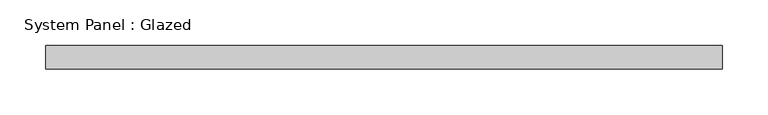
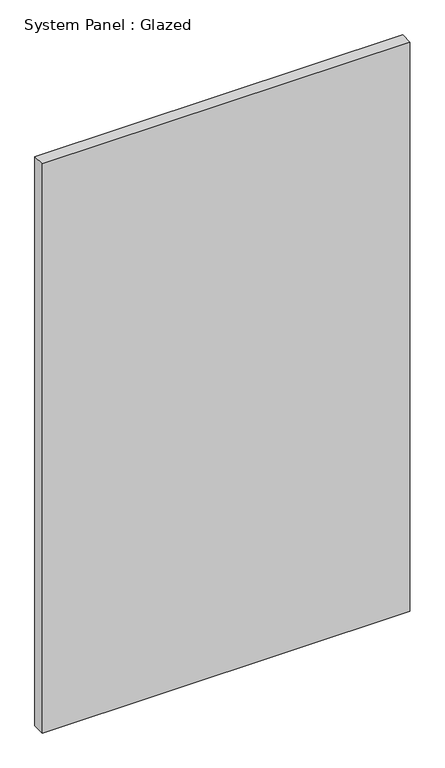
"""IFC4 building model written with IfcOpenShell, lengths in millimetres: plate geometry, System Panel : Glazed."""

from ifc_helpers import new_model, si_unit, origin, origin_with_axes, place, context, project, spatial, polyline, outline, extrude, source, transform, mapped, element, save


def system_panel_glazed_47c35fab(model_context):
    return source(origin(), model_context, "Body", "SweptSolid", [
        extrude(outline(polyline([(369.22075, 19.05), (-369.22075, 19.05), (-369.22075, 44.45), (369.22075, 44.45), (369.22075, 19.05)])), origin_with_axes(), (0.0, 0.0, 1.0), 1208.3415),
    ])


if __name__ == "__main__":
    model = new_model("IFC4")
    model_context = context("Model", 3, world=origin())
    ifc_project = project(units=[si_unit("LENGTHUNIT", "METRE", prefix="MILLI")], contexts=[model_context])
    site = spatial("IfcSite", under=ifc_project)
    building = spatial("IfcBuilding", under=site)
    placement = place(None, origin())
    system_panel_glazed_shape = system_panel_glazed_47c35fab(model_context)
    element("IfcPlate", 1, ObjectType="System Panel : Glazed", at=placement, inside=building, context=model_context, shape_type="MappedRepresentation", body=[
        mapped(system_panel_glazed_shape, transform((0.0, 0.0, 0.0), x_axis=(1.0, 0.0, 0.0), y_axis=(0.0, 1.0, 0.0), z_axis=(0.0, 0.0, 1.0))),
    ])
    save(model, "model.ifc")

# Revit data of these elements
# Type "System Panel : Glazed"
#   Construction Type Id = "GSP4R"
#   Analytic Construction = "1/8 in Pilkington single glazing"
#   Visual Light Transmittance = 0.9
#   Solar Heat Gain Coefficient = 0.86
#   Heat Transfer Coefficient (U) = 1.18115 BTU/(h·ft²·°F)
#   Define Thermal Properties by = 1
# Element 1 (IfcPlate, "System Panel : Glazed")
#   Materials on its faces: "Glass"
# Materials
#   "Glass": class "Glass", colour RGB 0 128 192, transparency 0.75, Description = "Soda Lime Glass", Cost = 0
